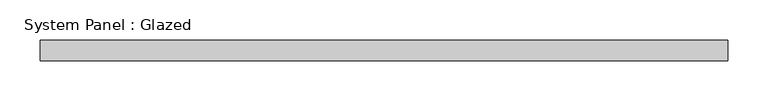
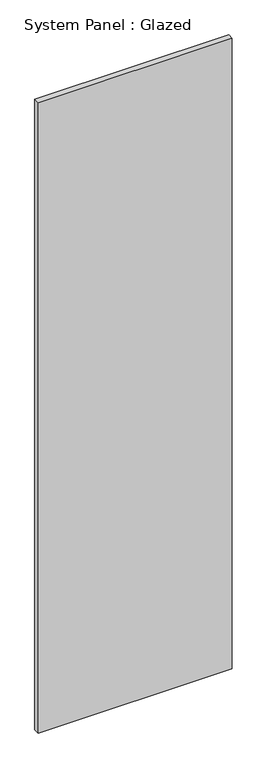
"""IFC4 building model written with IfcOpenShell, lengths in millimetres: plate geometry, System Panel : Glazed."""

from ifc_helpers import new_model, si_unit, origin, origin_with_axes, place, context, project, spatial, polyline, outline, extrude, source, transform, mapped, element, save


def system_panel_glazed_f0722de2(model_context):
    return source(origin(), model_context, "Body", "SweptSolid", [
        extrude(outline(polyline([(425.45, 19.05), (-425.45, 19.05), (-425.45, 44.45), (425.45, 44.45), (425.45, 19.05)])), origin_with_axes(), (0.0, 0.0, 1.0), 2921.0),
    ])


if __name__ == "__main__":
    model = new_model("IFC4")
    model_context = context("Model", 3, world=origin())
    ifc_project = project(units=[si_unit("LENGTHUNIT", "METRE", prefix="MILLI")], contexts=[model_context])
    site = spatial("IfcSite", under=ifc_project)
    building = spatial("IfcBuilding", under=site)
    placement = place(None, origin())
    system_panel_glazed_shape = system_panel_glazed_f0722de2(model_context)
    element("IfcPlate", 1, ObjectType="System Panel : Glazed", at=placement, inside=building, context=model_context, shape_type="MappedRepresentation", body=[
        mapped(system_panel_glazed_shape, transform((0.0, 0.0, 0.0), x_axis=(1.0, 0.0, 0.0), y_axis=(0.0, 1.0, 0.0), z_axis=(0.0, 0.0, 1.0))),
    ])
    save(model, "model.ifc")

# Revit data of these elements
# Type "System Panel : Glazed"
#   Construction Type Id = "GSP4R"
#   Analytic Construction = "1/8 in Pilkington single glazing"
#   Visual Light Transmittance = 0.9
#   Solar Heat Gain Coefficient = 0.86
#   Heat Transfer Coefficient (U) = 1.18115 BTU/(h·ft²·°F)
# Element 1 (IfcPlate, "System Panel : Glazed")
#   Materials on its faces: "Glass"
# Materials
#   "Glass": class "Glass", colour RGB 0 128 192, transparency 0.75, Description = "Soda Lime Glass", Cost = 0
